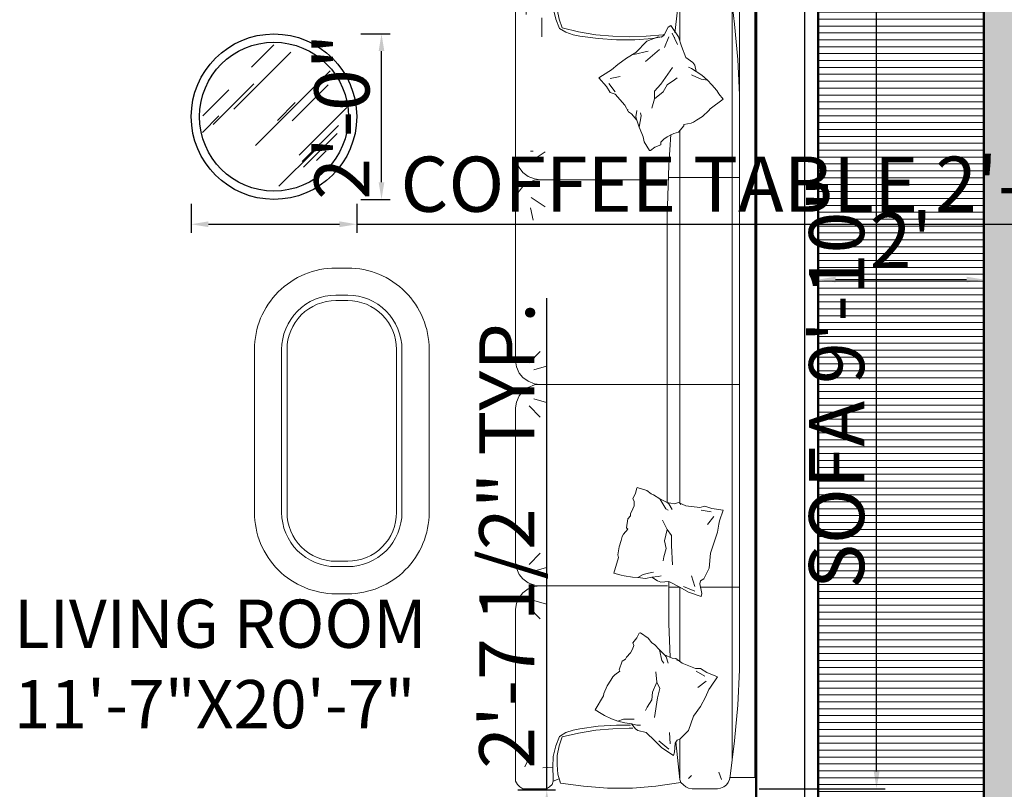
# Model space of a CAD drawing. Units: inches. Extents: x 1770 to 3141, y 984 to 1614.
# Tile 7 of 12: x 2124 to 2267, y 1407 to 1519. Entities that reach past the tile are written whole.
import ezdxf

# ---------------------------------------------------------------- set-up
doc = ezdxf.new("R2010")
doc.units = ezdxf.units.IN
for name, color, linetype, lineweight in [('A-ANNO-DIMS', 2, 'Continuous', 18), ('A-AREA-IDEN', 3, 'Continuous', 18), ('A-FLOR-PATT', 252, 'Continuous', 13), ('A-FURN', 8, 'Continuous', 18), ('A-GLAZ', 5, 'Continuous', 25), ('A-WALL', 7, 'Continuous', 50)]:
    doc.layers.add(name, color=color, linetype=linetype, lineweight=lineweight)
doc.layers.add('IFF-FURN', color=51, linetype='Continuous')
doc.styles.get("Standard").update_dxf_attribs({"font": 'arial.ttf'})
doc.dimstyles.new('ISO-25', dxfattribs={"dimtxt": 8, "dimasz": 2.5, "dimexe": 1.25, "dimexo": 0.625, "dimtad": 1, "dimdec": 1, "dimlunit": 3, "dimtxsty": 'Standard', "dimcen": 2.5, "dimclrt": 1, "dimadec": 0, "dimazin": 0, "dimtfac": 1, "dimtdec": 1, "dimtmove": 0, "dimatfit": 3, "dimfxl": 1, "dimarcsym": 0})

# ---------------------------------------------------------------- blocks, each defined once
blk = doc.blocks.new('sofa-42')
at = {"color": 0, "linetype": 'ByBlock'}
for p, q in [((-0.028, 0.939), (-0.038, 0.929)), ((-0.038, 0.929), (-0.028, 0.939)), ((-0.015, 0.947), (-0.028, 0.939)), ((-0.028, 0.939), (-0.015, 0.947)), ((-0.003, 0.947), (-0.015, 0.947)), ((-0.015, 0.947), (-0.003, 0.947)), ((0.665, 0.947), (-0.003, 0.947)), ((-0.003, 0.947), (0.665, 0.947)), ((0.687, 0.942), (0.665, 0.947)), ((0.687, 0.942), (0.665, 0.947)), ((0.712, 0.932), (0.687, 0.942)), ((0.712, 0.932), (0.687, 0.942)), ((0.827, 0.942), (0.802, 0.932)), ((0.802, 0.932), (0.827, 0.942)), ((0.85, 0.947), (0.827, 0.942)), ((0.827, 0.942), (0.85, 0.947)), ((1.462, 0.947), (0.85, 0.947)), ((0.85, 0.947), (1.462, 0.947)), ((1.484, 0.942), (1.462, 0.947)), ((1.484, 0.942), (1.462, 0.947)), ((1.509, 0.932), (1.484, 0.942)), ((1.509, 0.932), (1.484, 0.942)), ((1.599, 0.932), (1.624, 0.942)), ((1.624, 0.942), (1.599, 0.932)), ((1.624, 0.942), (1.647, 0.947)), ((1.647, 0.947), (1.624, 0.942)), ((1.647, 0.947), (2.272, 0.947)), ((2.272, 0.947), (1.647, 0.947)), ((2.297, 0.942), (2.272, 0.947)), ((2.297, 0.942), (2.272, 0.947)), ((2.319, 0.932), (2.297, 0.942)), ((2.319, 0.932), (2.297, 0.942)), ((2.434, 0.942), (2.412, 0.932)), ((2.412, 0.932), (2.434, 0.942)), ((2.457, 0.947), (2.434, 0.942)), ((2.434, 0.942), (2.457, 0.947)), ((3.127, 0.947), (2.457, 0.947)), ((2.457, 0.947), (3.127, 0.947)), ((3.139, 0.947), (3.127, 0.947)), ((3.139, 0.947), (3.127, 0.947)), ((3.152, 0.939), (3.139, 0.947)), ((3.152, 0.939), (3.139, 0.947)), ((3.162, 0.929), (3.152, 0.939)), ((3.162, 0.929), (3.152, 0.939)), ((-0.038, 0.929), (-0.045, 0.917)), ((-0.045, 0.917), (-0.038, 0.929)), ((-0.045, 0.917), (-0.045, 0.824)), ((-0.045, 0.917), (-0.045, 0.824)), ((0.042, 0.909), (0.087, 0.889)), ((0.73, 0.917), (0.712, 0.932)), ((0.73, 0.917), (0.712, 0.932)), ((0.745, 0.897), (0.73, 0.917)), ((0.745, 0.897), (0.73, 0.917)), ((0.755, 0.872), (0.745, 0.897)), ((0.755, 0.872), (0.745, 0.897)), ((0.77, 0.897), (0.76, 0.872)), ((0.76, 0.872), (0.77, 0.897)), ((0.785, 0.917), (0.77, 0.897)), ((0.77, 0.897), (0.785, 0.917)), ((0.802, 0.932), (0.785, 0.917)), ((0.785, 0.917), (0.802, 0.932)), ((1.527, 0.917), (1.509, 0.932)), ((1.527, 0.917), (1.509, 0.932)), ((1.542, 0.897), (1.527, 0.917)), ((1.542, 0.897), (1.527, 0.917)), ((1.552, 0.872), (1.542, 0.897)), ((1.552, 0.872), (1.542, 0.897)), ((1.557, 0.872), (1.567, 0.897)), ((1.567, 0.897), (1.557, 0.872)), ((1.567, 0.897), (1.582, 0.917)), ((1.582, 0.917), (1.567, 0.897)), ((1.582, 0.917), (1.599, 0.932)), ((1.599, 0.932), (1.582, 0.917)), ((2.337, 0.917), (2.319, 0.932)), ((2.337, 0.917), (2.319, 0.932)), ((2.352, 0.897), (2.337, 0.917)), ((2.352, 0.897), (2.337, 0.917)), ((2.362, 0.872), (2.352, 0.897)), ((2.362, 0.872), (2.352, 0.897)), ((2.377, 0.897), (2.367, 0.872)), ((2.367, 0.872), (2.377, 0.897)), ((2.392, 0.917), (2.377, 0.897)), ((2.377, 0.897), (2.392, 0.917)), ((2.412, 0.932), (2.392, 0.917)), ((2.392, 0.917), (2.412, 0.932)), ((3.067, 0.904), (3.017, 0.904)), ((3.169, 0.917), (3.162, 0.929)), ((3.169, 0.917), (3.162, 0.929)), ((3.169, 0.824), (3.169, 0.917)), ((3.169, 0.917), (3.169, 0.824)), ((0.672, 0.892), (0.627, 0.849)), ((0.7, 0.874), (0.685, 0.824)), ((0.757, 0.849), (0.755, 0.872)), ((0.757, 0.849), (0.755, 0.872)), ((0.76, 0.872), (0.757, 0.849)), ((0.757, 0.849), (0.76, 0.872)), ((0.815, 0.874), (0.83, 0.824)), ((0.842, 0.892), (0.887, 0.849)), ((1.469, 0.892), (1.424, 0.849)), ((1.497, 0.874), (1.482, 0.824)), ((1.554, 0.849), (1.552, 0.872)), ((1.554, 0.849), (1.552, 0.872)), ((1.554, 0.849), (1.557, 0.872)), ((1.557, 0.872), (1.554, 0.849)), ((1.612, 0.874), (1.627, 0.824)), ((1.639, 0.892), (1.684, 0.849)), ((2.252, 0.887), (2.204, 0.877)), ((2.294, 0.884), (2.257, 0.829)), ((2.364, 0.849), (2.362, 0.872)), ((2.364, 0.849), (2.362, 0.872)), ((2.367, 0.872), (2.364, 0.849)), ((2.364, 0.849), (2.367, 0.872)), ((2.437, 0.884), (2.474, 0.829)), ((2.477, 0.887), (2.477, 0.877)), ((-0.045, 0.824), (-0.038, 0.812)), ((-0.045, 0.824), (-0.038, 0.812)), ((0.04, 0.799), (0.037, 0.839)), ((0.757, 0.345), (0.757, 0.849)), ((1.554, 0.06), (1.554, 0.849)), ((2.364, 0.345), (2.364, 0.849)), ((3.004, 0.842), (2.929, 0.842)), ((3.162, 0.812), (3.169, 0.824)), ((3.169, 0.824), (3.162, 0.812)), ((-0.038, 0.812), (-0.028, 0.802)), ((-0.038, 0.812), (-0.028, 0.802)), ((-0.028, 0.802), (-0.015, 0.797)), ((-0.028, 0.802), (-0.015, 0.797)), ((-0.015, 0.797), (-0.0064, 0.7737)), ((-0.015, 0.797), (-0.003, 0.797)), ((-0.0064, 0.7737), (-0.015, 0.797)), ((0.04, 0.799), (-0.003, 0.797)), ((0.05, 0.782), (0.012, 0.779)), ((0.082, 0.797), (0.04, 0.799)), ((0.087, 0.782), (0.05, 0.782)), ((0.125, 0.787), (0.082, 0.797)), ((0.125, 0.774), (0.087, 0.782)), ((0.162, 0.772), (0.125, 0.787)), ((2.962, 0.772), (2.999, 0.787)), ((2.999, 0.787), (3.042, 0.797)), ((2.999, 0.774), (3.037, 0.782)), ((3.037, 0.782), (3.074, 0.782)), ((3.042, 0.797), (3.084, 0.799)), ((3.074, 0.782), (3.112, 0.779)), ((3.084, 0.799), (3.127, 0.797)), ((3.139, 0.797), (3.127, 0.797)), ((3.1318, 0.7734), (3.139, 0.797)), ((3.1318, 0.7734), (3.139, 0.797)), ((3.139, 0.797), (3.152, 0.802)), ((3.152, 0.802), (3.139, 0.797)), ((3.152, 0.802), (3.162, 0.812)), ((3.162, 0.812), (3.152, 0.802)), ((-0.023, 0.769), (-0.035, 0.677)), ((-0.023, 0.769), (-0.035, 0.677)), ((0.012, 0.779), (-0.023, 0.769)), ((-0.0064, 0.7737), (-0.023, 0.769)), ((0.16, 0.762), (0.125, 0.774)), ((0.175, 0.697), (0.16, 0.762)), ((0.177, 0.747), (0.162, 0.772)), ((0.187, 0.719), (0.177, 0.747)), ((2.937, 0.719), (2.947, 0.747)), ((2.947, 0.747), (2.962, 0.772)), ((2.949, 0.697), (2.964, 0.762)), ((2.964, 0.762), (2.999, 0.774)), ((3.112, 0.779), (3.147, 0.769)), ((3.147, 0.769), (3.1318, 0.7734)), ((3.159, 0.677), (3.147, 0.769)), ((3.147, 0.769), (3.159, 0.677)), ((0.192, 0.692), (0.187, 0.719)), ((2.932, 0.692), (2.937, 0.719)), ((-0.035, 0.677), (-0.043, 0.582)), ((-0.035, 0.677), (-0.043, 0.582)), ((0.187, 0.629), (0.175, 0.697)), ((0.202, 0.619), (0.192, 0.692)), ((2.922, 0.619), (2.932, 0.692)), ((2.937, 0.629), (2.949, 0.697)), ((3.167, 0.582), (3.159, 0.677)), ((3.159, 0.677), (3.167, 0.582)), ((0.192, 0.562), (0.187, 0.629)), ((0.267, 0.632), (0.252, 0.607)), ((0.322, 0.599), (0.267, 0.632)), ((2.932, 0.562), (2.937, 0.629)), ((0.207, 0.547), (0.202, 0.619)), ((0.245, 0.594), (0.232, 0.567)), ((0.252, 0.607), (0.245, 0.594)), ((0.332, 0.597), (0.322, 0.599)), ((0.362, 0.584), (0.332, 0.597)), ((2.732, 0.587), (2.709, 0.572)), ((2.767, 0.617), (2.732, 0.587)), ((2.792, 0.577), (2.767, 0.617)), ((2.917, 0.547), (2.922, 0.619)), ((-0.043, 0.582), (-0.043, 0.484)), ((-0.043, 0.582), (-0.043, 0.484)), ((0.195, 0.497), (0.192, 0.562)), ((0.207, 0.492), (0.207, 0.547)), ((0.232, 0.567), (0.222, 0.542)), ((0.385, 0.569), (0.362, 0.584)), ((0.397, 0.562), (0.385, 0.569)), ((0.405, 0.554), (0.397, 0.562)), ((0.42, 0.534), (0.405, 0.554)), ((0.807, 0.557), (0.8, 0.529)), ((0.87, 0.539), (0.807, 0.557)), ((2.702, 0.552), (2.659, 0.514)), ((2.709, 0.572), (2.702, 0.552)), ((2.744, 0.577), (2.712, 0.552)), ((2.764, 0.572), (2.772, 0.532)), ((2.799, 0.567), (2.792, 0.577)), ((2.819, 0.542), (2.799, 0.567)), ((2.917, 0.474), (2.917, 0.547)), ((2.929, 0.497), (2.932, 0.562)), ((3.167, 0.484), (3.167, 0.582)), ((3.167, 0.582), (3.167, 0.484)), ((0.215, 0.514), (0.212, 0.487)), ((0.222, 0.542), (0.215, 0.514)), ((0.222, 0.542), (0.23, 0.519)), ((0.23, 0.519), (0.23, 0.497)), ((0.425, 0.537), (0.42, 0.534)), ((0.46, 0.524), (0.425, 0.537)), ((0.467, 0.512), (0.46, 0.524)), ((0.475, 0.507), (0.467, 0.512)), ((0.492, 0.492), (0.475, 0.507)), ((0.797, 0.517), (0.792, 0.484)), ((0.8, 0.529), (0.797, 0.517)), ((0.88, 0.542), (0.87, 0.539)), ((0.912, 0.537), (0.88, 0.542)), ((0.937, 0.529), (0.912, 0.537)), ((0.952, 0.524), (0.937, 0.529)), ((0.962, 0.519), (0.952, 0.524)), ((0.982, 0.502), (0.962, 0.519)), ((0.987, 0.507), (0.982, 0.502)), ((1.022, 0.502), (0.987, 0.507)), ((2.659, 0.514), (2.632, 0.499)), ((2.844, 0.507), (2.819, 0.542)), ((2.867, 0.47), (2.844, 0.507)), ((-0.043, 0.484), (-0.035, 0.392)), ((-0.043, 0.484), (-0.035, 0.392)), ((0.192, 0.472), (0.185, 0.462)), ((0.212, 0.487), (0.192, 0.472)), ((0.195, 0.482), (0.195, 0.497)), ((0.207, 0.467), (0.212, 0.487)), ((0.23, 0.497), (0.23, 0.477)), ((0.507, 0.484), (0.492, 0.492)), ((0.522, 0.479), (0.507, 0.484)), ((0.532, 0.482), (0.522, 0.479)), ((0.552, 0.467), (0.532, 0.482)), ((0.792, 0.484), (0.79, 0.462)), ((1.035, 0.492), (1.022, 0.502)), ((1.042, 0.492), (1.035, 0.492)), ((1.062, 0.482), (1.042, 0.492)), ((1.074, 0.477), (1.062, 0.482)), ((1.092, 0.477), (1.074, 0.477)), ((1.102, 0.482), (1.092, 0.477)), ((1.124, 0.472), (1.102, 0.482)), ((1.144, 0.467), (1.124, 0.472)), ((2.624, 0.487), (2.599, 0.467)), ((2.599, 0.467), (2.612, 0.47)), ((2.612, 0.47), (2.637, 0.467)), ((2.632, 0.499), (2.624, 0.487)), ((2.637, 0.504), (2.642, 0.502)), ((2.872, 0.422), (2.859, 0.479)), ((2.912, 0.427), (2.867, 0.47)), ((2.922, 0.405), (2.917, 0.474)), ((2.932, 0.43), (2.929, 0.497)), ((3.159, 0.392), (3.167, 0.484)), ((3.167, 0.484), (3.159, 0.392)), ((0.177, 0.43), (0.145, 0.395)), ((0.185, 0.462), (0.177, 0.43)), ((0.207, 0.452), (0.207, 0.467)), ((0.277, 0.425), (0.265, 0.432)), ((0.55, 0.422), (0.572, 0.452)), ((0.57, 0.457), (0.552, 0.467)), ((0.572, 0.452), (0.57, 0.457)), ((0.79, 0.462), (0.787, 0.432)), ((0.787, 0.432), (0.792, 0.407)), ((0.79, 0.462), (0.802, 0.442)), ((0.802, 0.442), (0.807, 0.42)), ((1.134, 0.427), (1.147, 0.465)), ((1.147, 0.465), (1.144, 0.467)), ((2.514, 0.437), (2.479, 0.417)), ((2.534, 0.442), (2.514, 0.437)), ((2.547, 0.447), (2.534, 0.442)), ((2.572, 0.457), (2.547, 0.447)), ((2.599, 0.467), (2.572, 0.457)), ((2.572, 0.457), (2.617, 0.45)), ((2.617, 0.45), (2.629, 0.452)), ((2.879, 0.377), (2.832, 0.432)), ((2.937, 0.362), (2.932, 0.43)), ((-0.035, 0.392), (-0.02, 0.292)), ((-0.035, 0.392), (-0.02, 0.292)), ((0.145, 0.395), (0.117, 0.367)), ((0.237, 0.397), (0.315, 0.385)), ((0.307, 0.407), (0.277, 0.425)), ((0.337, 0.405), (0.307, 0.407)), ((0.377, 0.387), (0.337, 0.405)), ((0.377, 0.387), (0.417, 0.392)), ((0.505, 0.377), (0.525, 0.397)), ((0.525, 0.397), (0.532, 0.407)), ((0.532, 0.407), (0.55, 0.422)), ((0.792, 0.407), (0.777, 0.385)), ((0.795, 0.382), (0.792, 0.407)), ((0.807, 0.42), (0.812, 0.4)), ((1.102, 0.375), (1.117, 0.4)), ((1.117, 0.4), (1.122, 0.41)), ((1.122, 0.41), (1.134, 0.427)), ((2.479, 0.417), (2.479, 0.412)), ((2.479, 0.412), (2.492, 0.395)), ((2.492, 0.395), (2.502, 0.372)), ((2.684, 0.397), (2.647, 0.407)), ((2.684, 0.397), (2.712, 0.362)), ((2.714, 0.397), (2.684, 0.397)), ((2.742, 0.372), (2.714, 0.397)), ((2.929, 0.382), (2.912, 0.427)), ((2.927, 0.375), (2.922, 0.405)), ((3.132, 0.297), (3.159, 0.392)), ((3.159, 0.392), (3.132, 0.297)), ((0.117, 0.367), (0.087, 0.322)), ((0.112, 0.34), (0.145, 0.38)), ((0.315, 0.385), (0.352, 0.375)), ((0.352, 0.375), (0.377, 0.387)), ((0.462, 0.367), (0.452, 0.36)), ((0.505, 0.377), (0.462, 0.367)), ((0.472, 0.327), (0.485, 0.357)), ((0.485, 0.357), (0.477, 0.35)), ((0.485, 0.357), (0.505, 0.377)), ((0.777, 0.385), (0.772, 0.372)), ((0.772, 0.372), (0.775, 0.34)), ((0.797, 0.37), (0.795, 0.382)), ((0.872, 0.36), (0.857, 0.362)), ((0.905, 0.35), (0.872, 0.36)), ((0.935, 0.357), (0.905, 0.35)), ((0.98, 0.347), (0.935, 0.357)), ((0.98, 0.347), (1.017, 0.365)), ((1.062, 0.352), (1.057, 0.342)), ((1.102, 0.375), (1.062, 0.352)), ((1.087, 0.347), (1.102, 0.375)), ((2.502, 0.372), (2.512, 0.372)), ((2.512, 0.372), (2.524, 0.36)), ((2.524, 0.36), (2.534, 0.347)), ((2.712, 0.362), (2.739, 0.347)), ((2.807, 0.325), (2.742, 0.372)), ((2.929, 0.34), (2.887, 0.357)), ((2.927, 0.37), (2.929, 0.382)), ((2.934, 0.36), (2.927, 0.37)), ((2.967, 0.342), (2.934, 0.36)), ((2.939, 0.357), (2.937, 0.362)), ((0.14, 0.312), (-0.008, 0.297)), ((0.087, 0.322), (0.1, 0.317)), ((0.1, 0.317), (0.135, 0.315)), ((0.132, 0.335), (0.177, 0.337)), ((0.135, 0.315), (0.147, 0.307)), ((0.477, 0.35), (0.452, 0.342)), ((0.452, 0.287), (0.47, 0.312)), ((0.47, 0.312), (0.472, 0.327)), ((0.607, 0.34), (0.475, 0.335)), ((0.775, 0.34), (0.607, 0.34)), ((0.775, 0.34), (0.752, 0.297)), ((0.752, 0.297), (0.752, 0.34)), ((0.84, 0.325), (0.917, 0.33)), ((0.917, 0.33), (0.957, 0.33)), ((0.957, 0.33), (0.98, 0.347)), ((1.082, 0.34), (1.059, 0.327)), ((1.087, 0.347), (1.082, 0.34)), ((1.082, 0.317), (1.087, 0.347)), ((1.087, 0.302), (1.082, 0.317)), ((2.219, 0.347), (1.087, 0.347)), ((2.422, 0.34), (2.219, 0.347)), ((2.372, 0.06), (2.372, 0.34)), ((2.542, 0.332), (2.422, 0.34)), ((2.534, 0.347), (2.544, 0.325)), ((2.544, 0.325), (2.547, 0.32)), ((2.547, 0.32), (2.552, 0.302)), ((2.739, 0.347), (2.759, 0.317)), ((2.759, 0.317), (2.767, 0.307)), ((2.944, 0.327), (2.899, 0.305)), ((2.927, 0.317), (2.924, 0.317)), ((2.929, 0.302), (2.974, 0.332)), ((2.954, 0.315), (2.947, 0.317)), ((2.947, 0.315), (2.947, 0.317)), ((3.119, 0.297), (2.954, 0.315)), ((2.974, 0.332), (2.967, 0.342)), ((-0.03, 0.282), (-0.038, 0.272)), ((-0.03, 0.282), (-0.038, 0.272)), ((-0.02, 0.292), (-0.03, 0.282)), ((-0.02, 0.292), (-0.03, 0.282)), ((-0.008, 0.297), (-0.02, 0.292)), ((-0.008, 0.297), (0.15, 0.297)), ((0.005, 0.297), (-0.008, 0.297)), ((0.147, 0.307), (0.152, 0.295)), ((0.152, 0.295), (0.185, 0.262)), ((0.43, 0.235), (0.452, 0.287)), ((0.46, 0.297), (0.752, 0.297)), ((0.467, 0.307), (0.462, 0.307)), ((0.752, 0.297), (0.732, 0.262)), ((0.737, 0.237), (0.755, 0.282)), ((1.074, 0.272), (1.087, 0.302)), ((1.084, 0.297), (1.079, 0.292)), ((1.0855, 0.2985), (1.084, 0.297)), ((1.084, 0.297), (1.0848, 0.297)), ((1.084, 0.297), (2.372, 0.297)), ((1.0848, 0.297), (1.0855, 0.2985)), ((2.372, 0.297), (2.557, 0.297)), ((2.552, 0.302), (2.577, 0.28)), ((2.577, 0.28), (2.582, 0.28)), ((2.582, 0.28), (2.587, 0.252)), ((2.847, 0.272), (2.892, 0.29)), ((2.892, 0.29), (2.929, 0.302)), ((2.914, 0.297), (3.119, 0.297)), ((3.132, 0.297), (3.119, 0.297)), ((3.144, 0.292), (3.132, 0.297)), ((3.144, 0.292), (3.132, 0.297)), ((3.154, 0.282), (3.144, 0.292)), ((3.154, 0.282), (3.144, 0.292)), ((3.162, 0.272), (3.154, 0.282)), ((3.162, 0.272), (3.154, 0.282)), ((-0.043, 0.262), (-0.045, 0.247)), ((-0.043, 0.262), (-0.045, 0.247)), ((-0.045, 0.247), (-0.045, 0.147)), ((-0.045, 0.247), (-0.045, 0.147)), ((-0.038, 0.272), (-0.043, 0.262)), ((-0.038, 0.272), (-0.043, 0.262)), ((-0.005, 0.262), (0.007, 0.25)), ((0.185, 0.262), (0.242, 0.242)), ((0.242, 0.242), (0.28, 0.215)), ((0.43, 0.215), (0.43, 0.235)), ((0.732, 0.262), (0.715, 0.212)), ((0.755, 0.237), (0.797, 0.25)), ((1.067, 0.217), (1.074, 0.272)), ((2.587, 0.252), (2.592, 0.242)), ((2.592, 0.242), (2.599, 0.23)), ((2.769, 0.23), (2.779, 0.25)), ((2.804, 0.25), (2.792, 0.232)), ((2.792, 0.232), (2.817, 0.237)), ((2.809, 0.262), (2.804, 0.25)), ((2.817, 0.237), (2.827, 0.245)), ((2.827, 0.245), (2.847, 0.272)), ((3.109, 0.262), (3.074, 0.262)), ((3.167, 0.262), (3.162, 0.272)), ((3.167, 0.262), (3.162, 0.272)), ((3.169, 0.247), (3.167, 0.262)), ((3.169, 0.247), (3.167, 0.262)), ((3.169, 0.147), (3.169, 0.247)), ((3.169, 0.147), (3.169, 0.247)), ((0.28, 0.215), (0.317, 0.195)), ((0.317, 0.195), (0.347, 0.182)), ((0.38, 0.192), (0.355, 0.225)), ((0.4, 0.197), (0.42, 0.232)), ((0.415, 0.19), (0.43, 0.215)), ((0.715, 0.212), (0.727, 0.21)), ((0.727, 0.21), (0.765, 0.217)), ((0.752, 0.06), (0.752, 0.215)), ((0.765, 0.217), (0.777, 0.215)), ((0.777, 0.215), (0.785, 0.202)), ((0.785, 0.202), (0.827, 0.18)), ((1.05, 0.172), (1.057, 0.212)), ((1.064, 0.17), (1.072, 0.197)), ((1.072, 0.197), (1.067, 0.217)), ((2.599, 0.23), (2.614, 0.207)), ((2.614, 0.207), (2.637, 0.182)), ((2.757, 0.187), (2.762, 0.212)), ((2.757, 0.187), (2.777, 0.21)), ((2.762, 0.212), (2.769, 0.23)), ((2.777, 0.21), (2.792, 0.232)), ((0.347, 0.182), (0.357, 0.175)), ((0.357, 0.175), (0.397, 0.147)), ((0.397, 0.147), (0.415, 0.19)), ((0.827, 0.18), (0.887, 0.175)), ((0.887, 0.175), (0.93, 0.16)), ((0.93, 0.16), (0.97, 0.147)), ((1.032, 0.162), (1, 0.187)), ((1.057, 0.125), (1.064, 0.17)), ((2.637, 0.182), (2.644, 0.177)), ((2.644, 0.177), (2.682, 0.125)), ((2.717, 0.15), (2.739, 0.17)), ((2.739, 0.17), (2.757, 0.187)), ((-0.045, 0.147), (-0.043, 0.135)), ((-0.045, 0.147), (-0.043, 0.135)), ((-0.043, 0.135), (-0.038, 0.122)), ((-0.043, 0.135), (-0.038, 0.122)), ((-0.038, 0.122), (-0.03, 0.112)), ((-0.038, 0.122), (-0.03, 0.112)), ((-0.008, 0.132), (0.02, 0.142)), ((0.97, 0.147), (1.002, 0.142)), ((1.002, 0.142), (1.015, 0.14)), ((1.015, 0.14), (1.057, 0.125)), ((2.682, 0.125), (2.704, 0.142)), ((2.704, 0.142), (2.717, 0.15)), ((3.087, 0.142), (3.059, 0.155)), ((3.154, 0.112), (3.162, 0.122)), ((3.154, 0.112), (3.162, 0.122)), ((3.162, 0.122), (3.167, 0.135)), ((3.162, 0.122), (3.167, 0.135)), ((3.167, 0.135), (3.169, 0.147)), ((3.167, 0.135), (3.169, 0.147)), ((-0.03, 0.112), (-0.02, 0.105)), ((-0.03, 0.112), (-0.02, 0.105)), ((-0.02, 0.105), (-0.008, 0.1)), ((-0.02, 0.105), (-0.008, 0.1)), ((-0.008, 0.1), (0, 0.0982)), ((-0.008, 0.1), (0.005, 0.097)), ((0, 0.1), (0, 0)), ((0, 0.0982), (0, 0)), ((0.005, 0.097), (0.145, 0.08)), ((0.072, 0.09), (0.752, 0.09)), ((0.145, 0.08), (0.285, 0.067)), ((0.752, 0.09), (2.372, 0.09)), ((2.372, 0.09), (3.052, 0.09)), ((2.839, 0.067), (2.979, 0.08)), ((2.979, 0.08), (3.119, 0.097)), ((3.119, 0.097), (3.132, 0.1)), ((3.124, 0.0982), (3.132, 0.1)), ((3.124, 0.1), (3.124, 0)), ((3.124, 0), (3.124, 0.0982)), ((3.132, 0.1), (3.144, 0.105)), ((3.132, 0.1), (3.144, 0.105)), ((3.144, 0.105), (3.154, 0.112)), ((3.144, 0.105), (3.154, 0.112)), ((0.285, 0.067), (0.425, 0.06)), ((0.425, 0.06), (3.124, 0.06)), ((2.699, 0.06), (2.839, 0.067)), ((0, 0), (3.124, 0)), ((0, 0), (3.124, 0))]:
    blk.add_line(p, q, dxfattribs=at)
blk = doc.blocks.new('A$C384B067A')
for p, q in [((386.4, 723), (281.5, 618)), ((466.6, 689.5), (198.8, 421.7)), ((649.9, 600.8), (300.6, 251.5)), ((176.5, 513.1), (54.4, 390.9)), ((292.7, 540.9), (102, 350.2)), ((471.8, 367.3), (641.1, 536.6)), ((486.5, 453), (402.9, 369.4)), ((504.4, 207.2), (727.2, 430)), ((52.7, 313.8), (129.8, 391)), ((519.3, 177.3), (688.6, 346.5)), ((525.8, 151.5), (682.2, 307.9)), ((410.1, 61.5), (579.3, 230.8)), ((585.8, 181.5), (630.8, 226.5))]:
    blk.add_line(p, q)
at = {"layer": 'IFF-FURN'}
for p, q in [((386.4, 723), (281.5, 618)), ((386.4, 723), (281.5, 618)), ((386.4, 723), (281.5, 618)), ((466.6, 689.5), (198.8, 421.7)), ((466.6, 689.5), (198.8, 421.7)), ((466.6, 689.5), (198.8, 421.7)), ((649.9, 600.8), (300.6, 251.5)), ((649.9, 600.8), (300.6, 251.5)), ((649.9, 600.8), (300.6, 251.5)), ((176.5, 513.1), (54.4, 390.9)), ((176.5, 513.1), (54.4, 390.9)), ((176.5, 513.1), (54.4, 390.9)), ((292.7, 540.9), (102, 350.2)), ((292.7, 540.9), (102, 350.2)), ((292.7, 540.9), (102, 350.2)), ((471.8, 367.3), (641.1, 536.6)), ((471.8, 367.3), (641.1, 536.6)), ((471.8, 367.3), (641.1, 536.6)), ((486.5, 453), (402.9, 369.4)), ((486.5, 453), (402.9, 369.4)), ((486.5, 453), (402.9, 369.4)), ((504.4, 207.2), (727.2, 430)), ((504.4, 207.2), (727.2, 430)), ((504.4, 207.2), (727.2, 430)), ((52.7, 313.8), (129.8, 391)), ((52.7, 313.8), (129.8, 391)), ((52.7, 313.8), (129.8, 391)), ((519.3, 177.3), (688.6, 346.5)), ((519.3, 177.3), (688.6, 346.5)), ((519.3, 177.3), (688.6, 346.5)), ((525.8, 151.5), (682.2, 307.9)), ((525.8, 151.5), (682.2, 307.9)), ((525.8, 151.5), (682.2, 307.9)), ((410.1, 61.5), (579.3, 230.8)), ((410.1, 61.5), (579.3, 230.8)), ((410.1, 61.5), (579.3, 230.8)), ((585.8, 181.5), (630.8, 226.5)), ((585.8, 181.5), (630.8, 226.5)), ((585.8, 181.5), (630.8, 226.5))]:
    blk.add_line(p, q, dxfattribs=at)
for radius in [387.1, 348.4]:
    blk.add_circle((387.1, 387.1), radius, dxfattribs=at)
blk = doc.blocks.new('*D63')
at = {"layer": 'A-ANNO-DIMS', "color": 0, "lineweight": -2, "transparency": 16777216}
for p, q in [((2239.73, 1481.86), (2239.73, 1482.49)), ((2242.23, 1481.24), (2261.23, 1481.24)), ((2263.73, 1481.86), (2263.73, 1482.49))]:
    blk.add_line(p, q, dxfattribs=at)
at = {"layer": 'A-ANNO-DIMS', "color": 0, "transparency": 16777216}
for points in [[(2242.23, 1481.65), (2242.23, 1480.82), (2239.73, 1481.24)], [(2261.23, 1481.65), (2261.23, 1480.82), (2263.73, 1481.24)]]:
    blk.add_solid(points, dxfattribs=at)
at = {"layer": 'Defpoints', "color": 0, "transparency": 16777216}
for p in [(2239.73, 1481.24), (2263.73, 1481.24), (2263.73, 1481.24)]:
    blk.add_point(p, dxfattribs=at)
at = {"layer": 'A-ANNO-DIMS', "color": 0, "transparency": 16777216, "insert": (2251.73, 1485.88), "char_height": 8, "attachment_point": 5}
blk.add_mtext("2'", dxfattribs=at)
blk = doc.blocks.new('*D77')
at = {"layer": 'A-ANNO-DIMS', "color": 0, "lineweight": -2, "transparency": 16777216}
for p, q in [((2200.34, 1407.23), (2200.34, 1478.52)), ((2196.14, 1407.23), (2201.59, 1407.23)), ((2200.34, 1378.38), (2200.34, 1404.73)), ((2196.14, 1375.88), (2201.59, 1375.88))]:
    blk.add_line(p, q, dxfattribs=at)
at = {"layer": 'A-ANNO-DIMS', "color": 0, "transparency": 16777216}
for points in [[(2199.93, 1404.73), (2200.76, 1404.73), (2200.34, 1407.23)], [(2199.93, 1378.38), (2200.76, 1378.38), (2200.34, 1375.88)]]:
    blk.add_solid(points, dxfattribs=at)
at = {"layer": 'Defpoints', "color": 0, "transparency": 16777216}
for p in [(2195.51, 1407.23), (2200.34, 1407.23), (2195.51, 1375.88)]:
    blk.add_point(p, dxfattribs=at)
at = {"layer": 'A-ANNO-DIMS', "color": 1, "transparency": 16777216, "insert": (2195.58, 1444.13), "char_height": 8, "attachment_point": 5, "rotation": 90}
blk.add_mtext('2\'-7 1/2" TYP.', dxfattribs=at)
blk = doc.blocks.new('*D88')
at = {"layer": 'A-ANNO-DIMS', "color": 0, "lineweight": -2, "transparency": 16777216}
for p, q in [((2231.13, 1525.24), (2249.43, 1525.24)), ((2248.18, 1409.9), (2248.18, 1522.74)), ((2231.13, 1407.4), (2249.43, 1407.4))]:
    blk.add_line(p, q, dxfattribs=at)
at = {"layer": 'A-ANNO-DIMS', "color": 0, "transparency": 16777216}
for points in [[(2247.77, 1522.74), (2248.6, 1522.74), (2248.18, 1525.24)], [(2247.77, 1409.9), (2248.6, 1409.9), (2248.18, 1407.4)]]:
    blk.add_solid(points, dxfattribs=at)
at = {"layer": 'Defpoints', "color": 0, "transparency": 16777216}
for p in [(2230.51, 1525.24), (2248.18, 1525.24), (2230.51, 1407.4)]:
    blk.add_point(p, dxfattribs=at)
at = {"layer": 'A-ANNO-DIMS', "color": 1, "transparency": 16777216, "insert": (2243.42, 1466.32), "char_height": 8, "attachment_point": 5, "rotation": 90}
blk.add_mtext('SOFA 9\'-10"', dxfattribs=at)
blk = doc.blocks.new('*D90')
at = {"layer": 'A-ANNO-DIMS', "color": 0, "lineweight": -2, "transparency": 16777216}
for p, q in [((2148.77, 1492.24), (2148.77, 1488.01)), ((2172.77, 1492.24), (2172.77, 1488.01)), ((2151.27, 1489.26), (2170.27, 1489.26)), ((2172.77, 1489.26), (2284.63, 1489.26))]:
    blk.add_line(p, q, dxfattribs=at)
at = {"layer": 'A-ANNO-DIMS', "color": 0, "transparency": 16777216}
for points in [[(2151.27, 1489.68), (2151.27, 1488.84), (2148.77, 1489.26)], [(2170.27, 1489.68), (2170.27, 1488.84), (2172.77, 1489.26)]]:
    blk.add_solid(points, dxfattribs=at)
at = {"layer": 'Defpoints', "color": 0, "transparency": 16777216}
for p in [(2148.77, 1492.86), (2172.77, 1492.86), (2172.77, 1489.26)]:
    blk.add_point(p, dxfattribs=at)
at = {"layer": 'A-ANNO-DIMS', "color": 1, "transparency": 16777216, "insert": (2229.95, 1494.03), "char_height": 8, "attachment_point": 5}
blk.add_mtext('COFFEE TABLE 2\'-0"', dxfattribs=at)
blk = doc.blocks.new('*D91')
at = {"layer": 'A-ANNO-DIMS', "color": 0, "lineweight": -2, "transparency": 16777216}
for p, q in [((2173.39, 1516.86), (2177.62, 1516.86)), ((2176.37, 1495.36), (2176.37, 1514.36)), ((2173.39, 1492.86), (2177.62, 1492.86))]:
    blk.add_line(p, q, dxfattribs=at)
at = {"layer": 'A-ANNO-DIMS', "color": 0, "transparency": 16777216}
for points in [[(2175.95, 1514.36), (2176.78, 1514.36), (2176.37, 1516.86)], [(2175.95, 1495.36), (2176.78, 1495.36), (2176.37, 1492.86)]]:
    blk.add_solid(points, dxfattribs=at)
at = {"layer": 'Defpoints', "color": 0, "transparency": 16777216}
for p in [(2172.77, 1516.86), (2176.37, 1516.86), (2172.77, 1492.86)]:
    blk.add_point(p, dxfattribs=at)
at = {"layer": 'A-ANNO-DIMS', "color": 1, "transparency": 16777216, "insert": (2171.66, 1504.86), "char_height": 8, "attachment_point": 5, "rotation": 90}
blk.add_mtext('2\'-0"', dxfattribs=at)

msp = doc.modelspace()

# ---------------------------------------------------------------- hatches: boundary and pattern name
at = {"layer": 'A-FLOR-PATT'}
h = msp.add_hatch(color=256, dxfattribs=at)
h.dxf.hatch_style = 1
h.paths.add_polyline_path([(2384.73, 1565.18), (2263.73, 1565.18), (2263.73, 1347.18), (2333.73, 1347.18), (2333.73, 1356.18), (2272.73, 1356.18), (2272.73, 1556.18), (2375.73, 1556.18), (2375.73, 1347.18), (2384.73, 1347.18)])
h = msp.add_hatch(dxfattribs=at)
h.set_pattern_fill('_USER', color=256, pattern_type=0)
h.set_pattern_definition([(0, (0, 0), (0, 1), [])])
h.paths.add_polyline_path([(2408.73, 1561.18), (2384.73, 1561.18), (2384.73, 1347.18), (2375.73, 1347.18), (2263.73, 1347.18), (2263.73, 1561.18), (2239.73, 1561.18), (2239.73, 1300.18), (2408.73, 1300.18)])

# ---------------------------------------------------------------- linework, layer by layer
at = {"layer": 'A-FURN'}
for points in [[(2183.28, 1471.1), (2183.28, 1447.48, -0.414214), (2171.47, 1435.67), (2169.75, 1435.67, -0.414214), (2157.94, 1447.48), (2157.94, 1471.1, -0.414214), (2169.75, 1482.91), (2171.47, 1482.91, -0.414214)], [(2179.34, 1471.1), (2179.34, 1447.48, -0.414214), (2171.47, 1439.61), (2169.75, 1439.61, -0.414214), (2161.88, 1447.48), (2161.88, 1471.1, -0.414214), (2169.75, 1478.98), (2171.47, 1478.98, -0.414214)], [(2178.55, 1471.1), (2178.55, 1447.48, -0.414214), (2171.47, 1440.39), (2169.75, 1440.39, -0.414214), (2162.66, 1447.48), (2162.66, 1471.1, -0.414214), (2169.75, 1478.19), (2171.47, 1478.19, -0.414214)]]:
    msp.add_lwpolyline(points, format="xyb", close=True, dxfattribs=at)
at = {"layer": 'A-GLAZ'}
msp.add_line((2237.73, 1556.18), (2237.73, 1309.18), dxfattribs=at)
at = {"layer": 'A-WALL'}
for p, q in [((2239.73, 1565.18), (2239.73, 1288.18)), ((2263.73, 1565.18), (2263.73, 1347.18)), ((2230.73, 1556.18), (2230.73, 1309.18))]:
    msp.add_line(p, q, dxfattribs=at)

# ---------------------------------------------------------------- block references
at = {"layer": 'A-FURN', "xscale": 36.66436083614781, "yscale": 36.66436083614781, "zscale": 36.66436083614781, "rotation": 90}
msp.add_blockref('sofa-42', (2230.51, 1409.05), dxfattribs=at)
at = {"layer": 'A-FURN', "xscale": 0.031001591544, "yscale": 0.031001591544, "zscale": 0.031001591544}
msp.add_blockref('A$C384B067A', (2148.77, 1492.86), dxfattribs=at)

# ---------------------------------------------------------------- texts
at = {"layer": 'A-AREA-IDEN', "insert": (2123.04, 1434.83), "char_height": 7, "attachment_point": 1}
msp.add_mtext_dynamic_manual_height_columns('LIVING ROOM     11\'-7"X20\'-7"', width=86.9528, gutter_width=12.5, heights=[0], dxfattribs=at)

# ---------------------------------------------------------------- dimensions: what is measured, and where the dimension line sits
at = {"layer": 'A-ANNO-DIMS'}
for base, p1, p2, text, picture, middle in [((2248.18, 1525.24), (2230.51, 1407.4), (2230.51, 1525.24), 'SOFA <>', '*D88', (2243.42, 1466.32)), ((2200.3448, 1407.2305), (2195.5139, 1375.8824), (2195.5139, 1407.2305), '<> TYP.', '*D77', (2195.5834, 1444.1263))]:
    dim = msp.add_linear_dim(base=base, p1=p1, p2=p2, angle=90, text=text, dimstyle='ISO-25', override={"dimdec": 1, "dimrnd": 0, "dimzin": 1, "dimlunit": 4, "dimfrac": 2}, dxfattribs=at)
    dim.commit()
    dim.dimension.update_dxf_attribs({"geometry": picture, "text_midpoint": middle})
dim = msp.add_linear_dim(base=(2176.37, 1516.86), p1=(2172.77, 1492.86), p2=(2172.77, 1516.86), angle=90, dimstyle='ISO-25', override={"dimdec": 1, "dimrnd": 0, "dimzin": 1, "dimlunit": 4, "dimfrac": 2}, dxfattribs=at)
dim.commit()
dim.dimension.update_dxf_attribs({"geometry": '*D91', "text_midpoint": (2171.66, 1504.86)})
dim = msp.add_linear_dim(base=(2172.77, 1489.26), p1=(2148.77, 1492.86), p2=(2172.77, 1492.86), text='COFFEE TABLE <>', dimstyle='ISO-25', override={"dimdec": 1, "dimrnd": 0, "dimzin": 1, "dimlunit": 4, "dimfrac": 2}, dxfattribs=at)
dim.commit()
dim.dimension.update_dxf_attribs({"geometry": '*D90', "text_midpoint": (2229.95, 1494.03)})
dim = msp.add_linear_dim(base=(2263.73, 1481.24), p1=(2239.73, 1481.24), p2=(2263.73, 1481.24), dimstyle='ISO-25', override={"dimclrd": 0, "dimclre": 0, "dimclrt": 0}, dxfattribs=at)
dim.commit()
dim.dimension.update_dxf_attribs({"geometry": '*D63', "text_midpoint": (2251.73, 1485.88)})

doc.saveas('drawing.dxf')
